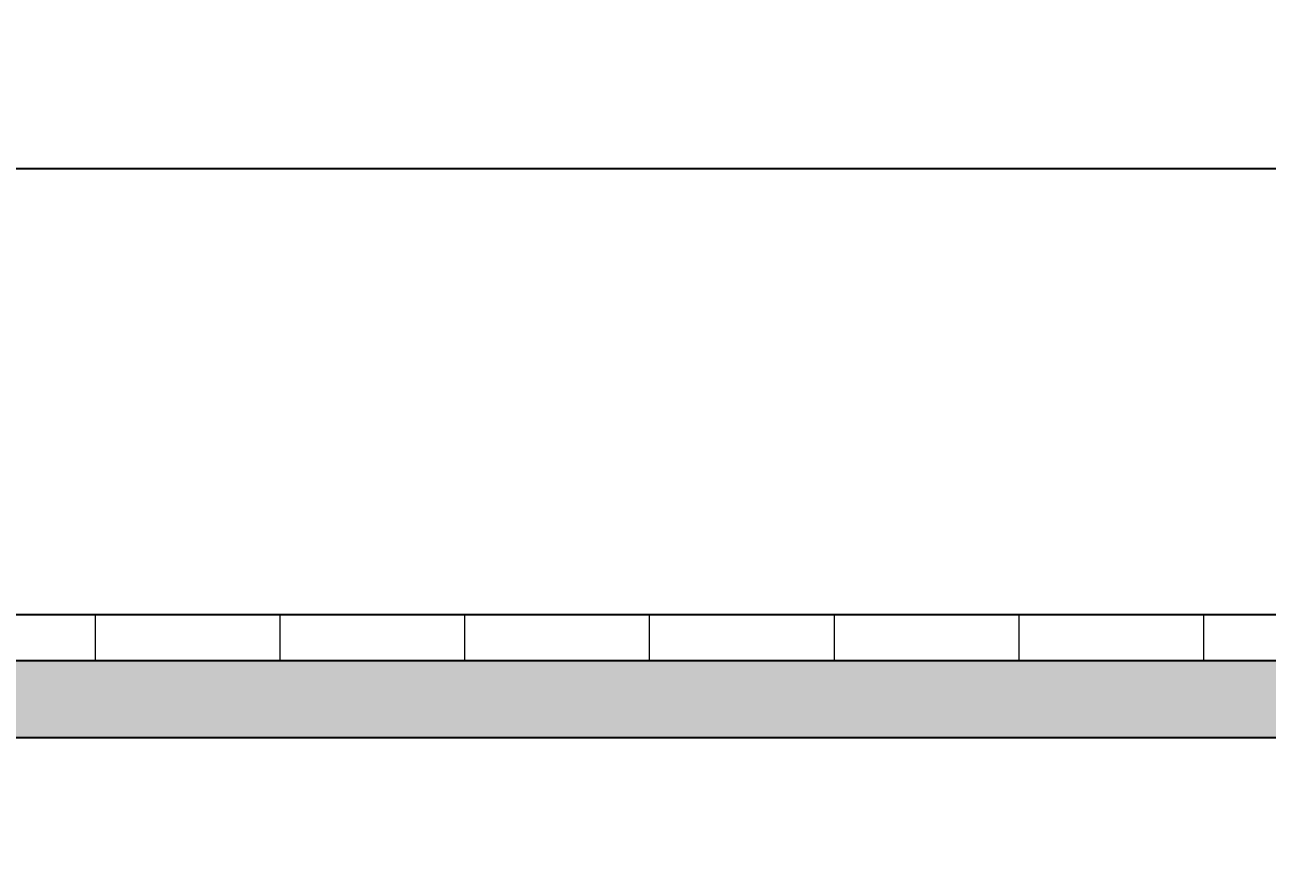
# Model space of a CAD drawing. Units: inches. Extents: x -301 to 715, y -607 to 364.
# Tile 44 of 141: x -17 to 64, y -370 to -315. Entities that reach past the tile are written whole.
import ezdxf

# ---------------------------------------------------------------- set-up
doc = ezdxf.new("R2010")
doc.units = ezdxf.units.IN
doc.header["$MEASUREMENT"] = 0
for name, color, linetype, lineweight in [('A-ANNO-DIMS', 2, 'Continuous', 18), ('A-SECT', 1, 'Continuous', 35), ('A-SECT-PATT', 8, 'Continuous', 13)]:
    doc.layers.add(name, color=color, linetype=linetype, lineweight=lineweight)
doc.styles.get("Standard").update_dxf_attribs({"font": 'arial.ttf'})
doc.dimstyles.get("Standard").update_dxf_attribs({"dimtxt": 0.18, "dimasz": 0.18, "dimexe": 0.18, "dimexo": 0.0625, "dimgap": 0.09, "dimtad": 0, "dimtih": 1, "dimtoh": 1, "dimdec": 1, "dimzin": 0, "dimdsep": 46, "dimlunit": 4, "dimtxsty": 'Standard', "dimcen": 0.09, "dimclrd": 3, "dimclre": 4, "dimclrt": 6, "dimadec": 0, "dimazin": 0, "dimtfac": 1, "dimtdec": 1, "dimtofl": 0, "dimtmove": 0, "dimatfit": 3, "dimfxl": 1, "dimtfill": 2, "dimtfillclr": 51, "dimtolj": 1, "dimtzin": 0, "dimarcsym": 0})

# ---------------------------------------------------------------- blocks, each defined once
blk = doc.blocks.new('*D175')
at = {"layer": 'A-ANNO-DIMS', "color": 4, "lineweight": -2, "transparency": 16777216}
for p, q in [((-199.282, -324.415), (-199.282, -292.467)), ((148.218, -324.415), (148.218, -292.467))]:
    blk.add_line(p, q, dxfattribs=at)
at = {"layer": 'A-ANNO-DIMS', "color": 3, "lineweight": -2, "transparency": 16777216}
for p, q in [((-199.102, -292.647), (-26.212, -292.647)), ((148.038, -292.647), (-24.852, -292.647))]:
    blk.add_line(p, q, dxfattribs=at)
at = {"layer": 'A-ANNO-DIMS', "color": 3, "transparency": 16777216}
for points in [[(-199.102, -292.617), (-199.102, -292.677), (-199.282, -292.647)], [(148.038, -292.617), (148.038, -292.677), (148.218, -292.647)]]:
    blk.add_solid(points, dxfattribs=at)
at = {"layer": 'Defpoints', "color": 0, "transparency": 16777216}
for p in [(148.218, -292.647), (-199.282, -324.477), (148.218, -324.477)]:
    blk.add_point(p, dxfattribs=at)
at = {"layer": 'A-ANNO-DIMS', "color": 6, "transparency": 16777216, "insert": (-25.532, -292.647), "char_height": 0.18, "attachment_point": 5, "bg_fill": 1, "box_fill_scale": 1.25, "bg_fill_color": 51, "bg_fill_transparency": 0}
blk.add_mtext('\\A1;28\'-11 1/2"', dxfattribs=at)
blk = doc.blocks.new('*D176')
at = {"layer": 'A-ANNO-DIMS', "color": 4, "lineweight": -2, "transparency": 16777216}
for p, q in [((148.28, -324.477), (215.605, -324.477)), ((-15.22, -540.477), (215.605, -540.477))]:
    blk.add_line(p, q, dxfattribs=at)
at = {"layer": 'A-ANNO-DIMS', "color": 3, "lineweight": -2, "transparency": 16777216}
for p, q in [((215.425, -324.657), (215.425, -432.296)), ((215.425, -540.297), (215.425, -432.659))]:
    blk.add_line(p, q, dxfattribs=at)
at = {"layer": 'A-ANNO-DIMS', "color": 3, "transparency": 16777216}
for points in [[(215.395, -324.657), (215.455, -324.657), (215.425, -324.477)], [(215.395, -540.297), (215.455, -540.297), (215.425, -540.477)]]:
    blk.add_solid(points, dxfattribs=at)
at = {"layer": 'Defpoints', "color": 0, "transparency": 16777216}
for p in [(148.218, -324.477), (-15.282, -540.477), (215.425, -540.477)]:
    blk.add_point(p, dxfattribs=at)
at = {"layer": 'A-ANNO-DIMS', "color": 6, "transparency": 16777216, "insert": (215.425, -432.477), "char_height": 0.18, "attachment_point": 5, "bg_fill": 1, "box_fill_scale": 1.25, "bg_fill_color": 51, "bg_fill_transparency": 0}
blk.add_mtext('\\A1;18\'-0"', dxfattribs=at)
blk = doc.blocks.new('*D189')
at = {"layer": 'A-ANNO-DIMS', "color": 4, "lineweight": -2, "transparency": 16777216}
for p, q in [((134.193, -353.477), (-266.112, -353.477)), ((134.193, -361.477), (-266.112, -361.477))]:
    blk.add_line(p, q, dxfattribs=at)
at = {"layer": 'A-ANNO-DIMS', "color": 3, "lineweight": -2, "transparency": 16777216}
for p, q in [((-265.932, -353.657), (-265.932, -357.296)), ((-265.932, -361.297), (-265.932, -357.659))]:
    blk.add_line(p, q, dxfattribs=at)
at = {"layer": 'A-ANNO-DIMS', "color": 3, "transparency": 16777216}
for points in [[(-265.962, -353.657), (-265.902, -353.657), (-265.932, -353.477)], [(-265.962, -361.297), (-265.902, -361.297), (-265.932, -361.477)]]:
    blk.add_solid(points, dxfattribs=at)
at = {"layer": 'Defpoints', "color": 0, "transparency": 16777216}
for p in [(134.255, -353.477), (-265.932, -361.477), (134.255, -361.477)]:
    blk.add_point(p, dxfattribs=at)
at = {"layer": 'A-ANNO-DIMS', "color": 6, "transparency": 16777216, "insert": (-265.932, -357.477), "char_height": 0.18, "attachment_point": 5, "bg_fill": 1, "box_fill_scale": 1.25, "bg_fill_color": 51, "bg_fill_transparency": 0}
blk.add_mtext('\\A1;0\'-8"', dxfattribs=at)

msp = doc.modelspace()

# ---------------------------------------------------------------- hatches: boundary and pattern name
at = {"layer": 'A-SECT-PATT'}
h = msp.add_hatch(dxfattribs=at)
h.set_pattern_fill('ANSI31', color=256, scale=96, angle=45, style=0)
h.paths.add_polyline_path([(-185.282, -356.477), (134.255, -356.477), (134.255, -353.477), (-185.282, -353.477)])
h = msp.add_hatch(dxfattribs=at)
h.set_pattern_fill('AR-CONC', color=256, scale=0.5)
h.set_pattern_definition([(50, (10.3213, 33.8764), (3.586301, -0.31376), [0.375, -4.125]), (355, (10.3213, 33.8764), (-0.693757, 3.76096), [0.3, -3.3]), (100.45144, (10.62, 33.8502), (2.892544, 3.4472), [0.3187, -3.50571]), (46.1842, (10.3213, 34.8764), (5.336207, -0.827596), [0.5625, -6.1875]), (96.6356, (10.766, 34.8074), (4.67331, 4.870593), [0.47805, -5.25857]), (351.1842, (10.321, 34.8764), (4.67331, 4.870593), [0.45, -4.95]), (21, (10.8213, 34.6264), (2.984535, -2.013094), [0.375, -4.125]), (326, (10.8213, 34.6264), (1.216577, 3.62575), [0.3, -3.3]), (71.45144, (11.07, 34.4586), (4.201112, 1.612656), [0.3187, -3.50571]), (37.5, (10.3213, 33.8764), (0.0607993, 1.6644693), [0, -3.26, 0, -3.35, 0, -3.3125]), (7.5, (10.3213, 33.8764), (1.3153477, 1.9720586), [0, -1.91, 0, -3.185, 0, -1.2625]), (327.5, (9.2063, 33.8764), (2.6691122, -0.1127744), [0, -1.25, 0, -3.9, 0, -5.175]), (317.5, (8.7063, 33.8764), (2.915931, 0.500525), [0, -1.625, 0, -2.59, 0, -3.675])])
h.paths.add_polyline_path([(-56.282, -535.477), (-61.282, -535.477), (-61.282, -540.477), (-15.282, -540.477), (-15.282, -535.477), (-20.282, -535.477)])
h.paths.add_polyline_path([(119.255, -535.477), (114.255, -535.477), (114.255, -540.477), (163.255, -540.477), (163.255, -535.477), (158.255, -535.477)])
h.paths.add_polyline_path([(-206.282, -471.477), (-209.282, -471.477), (-209.282, -481.477), (-206.282, -481.477), (-194.282, -481.477), (-194.282, -471.477)])
h.paths.add_polyline_path([(-41.282, -481.477), (-41.282, -471.477), (-185.282, -471.477), (-185.282, -481.477), (-180.282, -481.477)])
h.paths.add_polyline_path([(134.255, -481.477), (134.255, -471.477), (-35.282, -471.477), (-35.282, -481.477), (-30.282, -481.477)])
h.paths.add_polyline_path([(155.218, -481.477), (158.218, -481.477), (158.218, -471.477), (153.218, -471.477), (143.218, -471.477), (143.218, -481.477), (148.255, -481.477)])
h.paths.add_polyline_path([(-193.88, -356.477), (-193.904, -361.477), (143.218, -361.477), (143.218, -356.477)])

# ---------------------------------------------------------------- linework, layer by layer
at = {"layer": 'A-SECT'}
for p, q in [((-185.282, -324.477), (134.255, -324.477)), ((-194.282, -353.477), (143.218, -353.477)), ((-194.282, -356.477), (143.218, -356.477)), ((-194.282, -361.477), (143.218, -361.477))]:
    msp.add_line(p, q, dxfattribs=at)

# ---------------------------------------------------------------- dimensions: what is measured, and where the dimension line sits
at = {"layer": 'A-ANNO-DIMS'}
dim = msp.add_linear_dim(base=(148.218, -292.647), p1=(-199.282, -324.477), p2=(148.218, -324.477), dimstyle='Standard', override={"dimdec": 1, "dimlfac": 1, "dimrnd": 0, "dimzin": 1, "dimdsep": 46, "dimlunit": 4, "dimfrac": 2}, dxfattribs=at)
dim.commit()
dim.dimension.update_dxf_attribs({"geometry": '*D175', "text_midpoint": (-25.532, -292.647)})
for base, p1, p2, picture, middle in [((215.425, -540.477), (148.218, -324.477), (-15.282, -540.477), '*D176', (215.425, -432.477)), ((-265.932, -361.477), (134.255, -353.477), (134.255, -361.477), '*D189', (-265.932, -357.477))]:
    dim = msp.add_linear_dim(base=base, p1=p1, p2=p2, angle=90, dimstyle='Standard', override={"dimdec": 1, "dimlfac": 1, "dimrnd": 0, "dimzin": 1, "dimdsep": 46, "dimlunit": 4, "dimfrac": 2}, dxfattribs=at)
    dim.commit()
    dim.dimension.update_dxf_attribs({"geometry": picture, "text_midpoint": middle})

doc.saveas('drawing.dxf')
